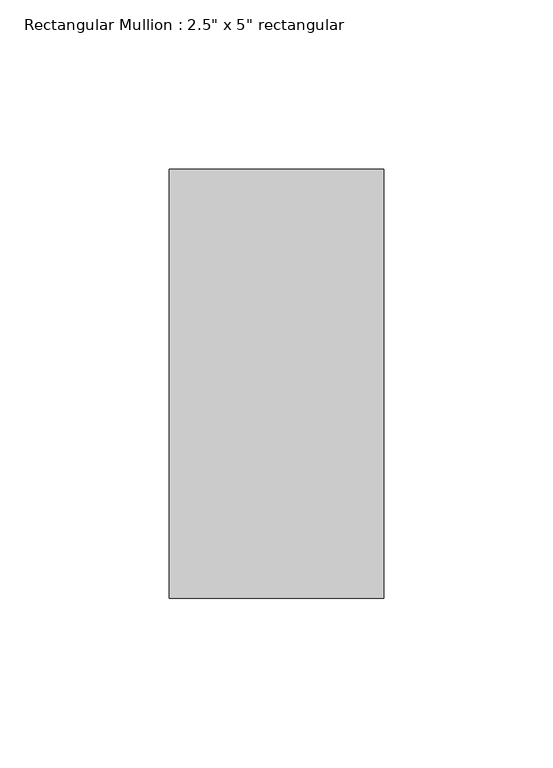
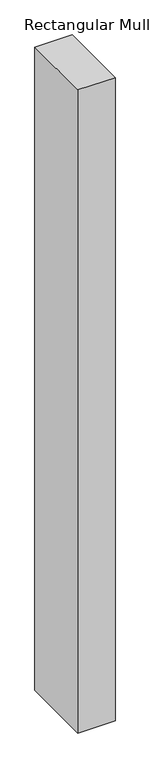
"""IFC4 building model written with IfcOpenShell, lengths in millimetres: member geometry."""

from ifc_helpers import new_model, si_unit, frame, origin, place, context, project, spatial, polyline, outline, extrude, source, transform, mapped, element, save


def member_6b401d40(model_context):
    return source(origin(), model_context, "Body", "SweptSolid", [
        extrude(outline(polyline([(0.0, 63.5), (0.0, -63.5), (-63.5, -63.5), (-63.5, 63.5), (0.0, 63.5)])), frame((0.0, 0.0, -1160.78), z_axis=(0.0, 0.0, 1.0), x_axis=(1.0, 0.0, 0.0)), (0.0, 0.0, 1.0), 1160.78),
    ])


if __name__ == "__main__":
    model = new_model("IFC4")
    model_context = context("Model", 3, world=origin())
    ifc_project = project(units=[si_unit("LENGTHUNIT", "METRE", prefix="MILLI")], contexts=[model_context])
    site = spatial("IfcSite", under=ifc_project)
    building = spatial("IfcBuilding", under=site)
    placement = place(None, origin())
    member_shape = member_6b401d40(model_context)
    element("IfcMember", 1, ObjectType="Rectangular Mullion : 2.5\" x 5\" rectangular", at=placement, inside=building, context=model_context, shape_type="MappedRepresentation", body=[
        mapped(member_shape, transform((0.0, 0.0, 0.0), x_axis=(1.0, 0.0, 0.0), y_axis=(0.0, 1.0, 0.0), z_axis=(0.0, 0.0, 1.0))),
    ])
    save(model, "model.ifc")

# Revit data of these elements
# Type "Rectangular Mullion : 2.5\" x 5\" rectangular"
#   built-in parameter 1007304 = 0.416667 (stored number, unit not read)
#   built-in parameter 1007301 = 0.104167 (stored number, unit not read)
#   built-in parameter 1007300 = 0.104167 (stored number, unit not read)
# Element 1 (IfcMember, "Rectangular Mullion : 2.5\" x 5\" rectangular")
#   Materials on its faces: "Aluminum"
# Materials
#   "Aluminum": class "Metal", colour RGB 247 247 247, transparency 0, Description = "Aluminum 6061", Cost = 0
